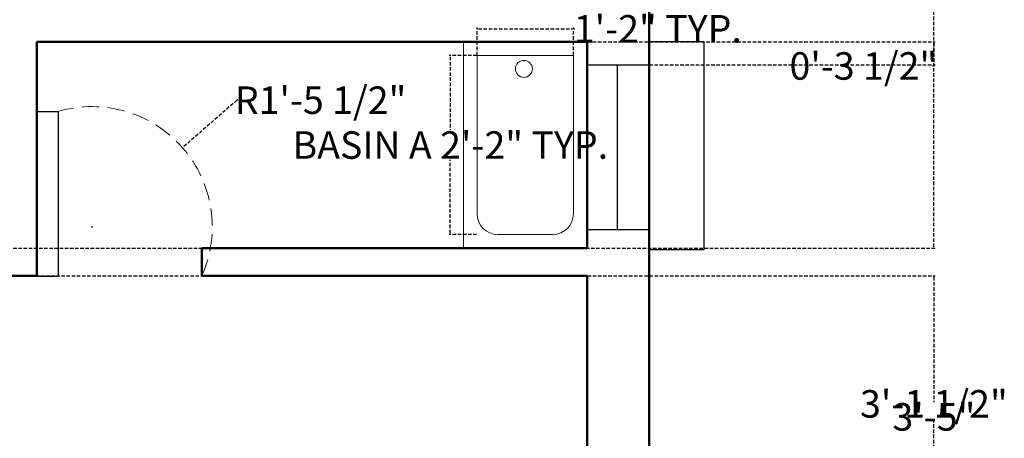
# Model space of a CAD drawing. Units: inches. Extents: x 513 to 1142, y 396 to 927.
# Tile 27 of 31: x 998 to 1142, y 614 to 674. Entities that reach past the tile are written whole.
import ezdxf

# ---------------------------------------------------------------- set-up
doc = ezdxf.new("R2010")
doc.units = ezdxf.units.IN
doc.header["$MEASUREMENT"] = 0
doc.linetypes.add('DASHED', pattern=[0.75, 0.5, -0.25])
for name, color, linetype, lineweight in [('A-ANNO-DIMS', 2, 'DASHED', 18), ('A-DOOR', 4, 'Continuous', 25), ('A-DOOR-SWNG', 4, 'DASHED', 13), ('A-FLOR-FIXT', 92, 'Continuous', 18), ('A-WALL', 7, 'Continuous', 50), ('windows', 172, 'Continuous', 25)]:
    doc.layers.add(name, color=color, linetype=linetype, lineweight=lineweight)
doc.styles.get("Standard").update_dxf_attribs({"font": 'arial.ttf'})
doc.dimstyles.get("Standard").update_dxf_attribs({"dimtxt": 4, "dimasz": 0.18, "dimexe": 0.18, "dimexo": 0.0625, "dimgap": 0.09, "dimtad": 0, "dimtih": 1, "dimtoh": 1, "dimdec": 0, "dimrnd": 6, "dimzin": 0, "dimdsep": 46, "dimlunit": 3, "dimtxsty": 'Standard', "dimcen": 0.09, "dimadec": 0, "dimazin": 0, "dimtfac": 1, "dimtdec": 0, "dimtofl": 0, "dimtmove": 0, "dimatfit": 3, "dimfxl": 1, "dimtolj": 1, "dimtzin": 0, "dimarcsym": 0})

# ---------------------------------------------------------------- blocks, each defined once
blk = doc.blocks.new('WIN-24IN')
blk.add_line((0, 4.39), (24, 4.39))
blk.add_lwpolyline([(24, 0), (0, 0), (0, 9), (24, 9)], close=True)
blk = doc.blocks.new('DOOR-LEAF-24IN')
blk.add_lwpolyline([(3, 24), (3, 0), (0, 0), (0, 24)], close=True)
blk = doc.blocks.new('BASIN-BOWL-14X26')
for p, q in [((0, 3), (0, 26)), ((0, 26), (14, 26)), ((14, 3), (14, 26)), ((3, 0), (11, 0))]:
    blk.add_line(p, q)
for centre, start, end in [((3, 3), 180, 270), ((11, 3), 270, 0)]:
    blk.add_arc(centre, 3, start, end)
blk = doc.blocks.new('*D131')
at = {"layer": 'A-ANNO-DIMS', "color": 0, "lineweight": -2, "transparency": 16777216}
for p, q in [((1064.93, 669.16), (1060.92, 669.16)), ((1061.1, 668.98), (1061.1, 658.32)), ((1061.1, 643.34), (1061.1, 654)), ((1064.93, 643.16), (1060.92, 643.16))]:
    blk.add_line(p, q, dxfattribs=at)
at = {"layer": 'A-ANNO-DIMS', "color": 0, "transparency": 16777216}
for points in [[(1061.07, 668.98), (1061.13, 668.98), (1061.1, 669.16)], [(1061.07, 643.34), (1061.13, 643.34), (1061.1, 643.16)]]:
    blk.add_solid(points, dxfattribs=at)
at = {"layer": 'Defpoints', "color": 0, "transparency": 16777216}
for p in [(1061.1, 669.16), (1065, 669.16), (1065, 643.16)]:
    blk.add_point(p, dxfattribs=at)
at = {"layer": 'A-ANNO-DIMS', "color": 0, "transparency": 16777216, "insert": (1061.1, 656.16), "char_height": 4, "attachment_point": 5}
blk.add_mtext('\\A1;BASIN A 2\'-2" TYP.', dxfattribs=at)
blk = doc.blocks.new('*D132')
at = {"layer": 'A-ANNO-DIMS', "color": 0, "lineweight": -2, "transparency": 16777216}
for p, q in [((1065, 669.22), (1065, 673.24)), ((1065.18, 673.06), (1078.82, 673.06)), ((1079, 669.22), (1079, 673.24)), ((1079, 673.06), (1079.18, 673.06))]:
    blk.add_line(p, q, dxfattribs=at)
at = {"layer": 'A-ANNO-DIMS', "color": 0, "transparency": 16777216}
for points in [[(1065.18, 673.09), (1065.18, 673.03), (1065, 673.06)], [(1078.82, 673.09), (1078.82, 673.03), (1079, 673.06)]]:
    blk.add_solid(points, dxfattribs=at)
at = {"layer": 'Defpoints', "color": 0, "transparency": 16777216}
for p in [(1079, 673.06), (1065, 669.16), (1079, 669.16)]:
    blk.add_point(p, dxfattribs=at)
at = {"layer": 'A-ANNO-DIMS', "color": 0, "transparency": 16777216, "insert": (1091.27, 673.06), "char_height": 4, "attachment_point": 5}
blk.add_mtext('\\A1;1\'-2" TYP.', dxfattribs=at)
blk = doc.blocks.new('*D149')
at = {"layer": 'A-ANNO-DIMS', "color": 0, "lineweight": -2, "transparency": 16777216}
for p, q in [((840.06, 770.16), (1131.58, 770.16)), ((1131.4, 769.98), (1131.4, 707.79)), ((1131.4, 641.34), (1131.4, 703.53)), ((840.06, 641.16), (1131.58, 641.16))]:
    blk.add_line(p, q, dxfattribs=at)
at = {"layer": 'A-ANNO-DIMS', "color": 0, "transparency": 16777216}
for points in [[(1131.37, 769.98), (1131.43, 769.98), (1131.4, 770.16)], [(1131.37, 641.34), (1131.43, 641.34), (1131.4, 641.16)]]:
    blk.add_solid(points, dxfattribs=at)
at = {"layer": 'Defpoints', "color": 0, "transparency": 16777216}
for p in [(840, 770.16), (1131.4, 770.16), (840, 641.16)]:
    blk.add_point(p, dxfattribs=at)
at = {"layer": 'A-ANNO-DIMS', "color": 0, "transparency": 16777216, "insert": (1131.4, 705.66), "char_height": 4, "attachment_point": 5}
blk.add_mtext('\\A1;10\'-9"', dxfattribs=at)
blk = doc.blocks.new('*D162')
at = {"layer": 'A-ANNO-DIMS', "color": 0, "lineweight": -2, "transparency": 16777216}
for p, q in [((1081.06, 637.16), (1131.58, 637.16)), ((1131.4, 636.98), (1131.4, 620.68)), ((1131.4, 600.06), (1131.4, 616.36)), ((1080.99, 599.88), (1131.58, 599.88))]:
    blk.add_line(p, q, dxfattribs=at)
at = {"layer": 'A-ANNO-DIMS', "color": 0, "transparency": 16777216}
for points in [[(1131.37, 636.98), (1131.43, 636.98), (1131.4, 637.16)], [(1131.37, 600.06), (1131.43, 600.06), (1131.4, 599.88)]]:
    blk.add_solid(points, dxfattribs=at)
at = {"layer": 'Defpoints', "color": 0, "transparency": 16777216}
for p in [(1081, 637.16), (1080.93, 599.88), (1131.4, 599.88)]:
    blk.add_point(p, dxfattribs=at)
at = {"layer": 'A-ANNO-DIMS', "color": 0, "transparency": 16777216, "insert": (1131.4, 618.52), "char_height": 4, "attachment_point": 5}
blk.add_mtext('\\A1;3\'-1 1/2"', dxfattribs=at)
blk = doc.blocks.new('*D166')
at = {"layer": 'A-ANNO-DIMS', "color": 0, "lineweight": -2, "transparency": 16777216}
for p, q in [((1081.06, 671.16), (1131.58, 671.16)), ((1131.4, 670.98), (1131.4, 668.02)), ((1081.03, 667.84), (1131.58, 667.84)), ((1131.4, 667.66), (1131.22, 667.66)), ((1131.4, 667.84), (1131.4, 667.66))]:
    blk.add_line(p, q, dxfattribs=at)
at = {"layer": 'A-ANNO-DIMS', "color": 0, "transparency": 16777216}
for points in [[(1131.37, 670.98), (1131.43, 670.98), (1131.4, 671.16)], [(1131.37, 668.02), (1131.43, 668.02), (1131.4, 667.84)]]:
    blk.add_solid(points, dxfattribs=at)
at = {"layer": 'Defpoints', "color": 0, "transparency": 16777216}
for p in [(1081, 671.16), (1080.97, 667.84), (1131.4, 667.84)]:
    blk.add_point(p, dxfattribs=at)
at = {"layer": 'A-ANNO-DIMS', "color": 0, "transparency": 16777216, "insert": (1121.15, 667.66), "char_height": 4, "attachment_point": 5}
blk.add_mtext('\\A1;0\'-3 1/2"', dxfattribs=at)
blk = doc.blocks.new('*D173')
at = {"layer": 'A-ANNO-DIMS', "color": 0, "lineweight": -2, "transparency": 16777216}
for p, q in [((904.06, 637.16), (1131.58, 637.16)), ((1131.4, 636.98), (1131.4, 618.76)), ((1131.4, 596.27), (1131.4, 614.49)), ((904.06, 596.09), (1131.58, 596.09))]:
    blk.add_line(p, q, dxfattribs=at)
at = {"layer": 'A-ANNO-DIMS', "color": 0, "transparency": 16777216}
for points in [[(1131.37, 636.98), (1131.43, 636.98), (1131.4, 637.16)], [(1131.37, 596.27), (1131.43, 596.27), (1131.4, 596.09)]]:
    blk.add_solid(points, dxfattribs=at)
at = {"layer": 'Defpoints', "color": 0, "transparency": 16777216}
for p in [(904, 637.16), (1131.4, 637.16), (904, 596.09)]:
    blk.add_point(p, dxfattribs=at)
at = {"layer": 'A-ANNO-DIMS', "color": 0, "transparency": 16777216, "insert": (1131.4, 616.63), "char_height": 4, "attachment_point": 5}
blk.add_mtext('\\A1;3\'-5"', dxfattribs=at)
blk = doc.blocks.new('*D189')
at = {"layer": 'A-ANNO-DIMS', "color": 0, "lineweight": -2, "transparency": 16777216}
for p, q in [((1030.08, 662.68), (1022.31, 655.89)), ((1030.26, 662.68), (1030.08, 662.68)), ((1008.92, 644.26), (1009.1, 644.26)), ((1009.01, 644.17), (1009.01, 644.35))]:
    blk.add_line(p, q, dxfattribs=at)
at = {"layer": 'A-ANNO-DIMS', "color": 0, "transparency": 16777216}
blk.add_solid([(1022.29, 655.91), (1022.33, 655.87), (1022.18, 655.77)], dxfattribs=at)
at = {"layer": 'Defpoints', "color": 0, "transparency": 16777216}
for p in [(1022.18, 655.77), (1009.01, 644.26)]:
    blk.add_point(p, dxfattribs=at)
at = {"layer": 'A-ANNO-DIMS', "color": 0, "transparency": 16777216, "insert": (1042.24, 662.68), "char_height": 4, "attachment_point": 5}
blk.add_mtext('\\A1;R1\'-5 1/2"', dxfattribs=at)

msp = doc.modelspace()

# ---------------------------------------------------------------- linework, layer by layer
at = {"layer": 'A-DOOR-SWNG', "ltscale": 5}
msp.add_arc((1009.01, 644.26), 17.49, 336.0483, 106.2786, dxfattribs=at)
at = {"layer": 'A-FLOR-FIXT'}
msp.add_line((1063, 641.16), (1063, 671.16), dxfattribs=at)
msp.add_circle((1071.8, 667.23), 1.23, dxfattribs=at)
at = {"layer": 'A-WALL'}
for p, q in [((1090, 431.16), (1090, 879.16)), ((1001, 637.16), (1001, 671.16)), ((1001, 671.16), (1081, 671.16)), ((1081, 641.16), (1081, 671.16)), ((1025, 637.16), (1025, 641.16)), ((1025, 641.16), (1081, 641.16)), ((949, 637.16), (1001, 637.16)), ((1025, 637.16), (1081, 637.16)), ((1081, 497.16), (1081, 637.16))]:
    msp.add_line(p, q, dxfattribs=at)
at = {"layer": 'windows'}
for p, q in [((1098, 671.16), (1090, 671.16)), ((1098, 640.92), (1098, 671.16)), ((1098, 640.92), (1090, 640.92))]:
    msp.add_line(p, q, dxfattribs=at)

# ---------------------------------------------------------------- block references
at = {"layer": 'A-DOOR'}
msp.add_blockref('DOOR-LEAF-24IN', (1001.11, 637.05), dxfattribs=at)
at = {"layer": 'A-FLOR-FIXT'}
msp.add_blockref('BASIN-BOWL-14X26', (1064.99, 643.16), dxfattribs=at)
at = {"layer": 'windows', "rotation": 270.0000000000006}
msp.add_blockref('WIN-24IN', (1080.97, 667.84), dxfattribs=at)

# ---------------------------------------------------------------- dimensions: what is measured, and where the dimension line sits
at = {"layer": 'A-ANNO-DIMS'}
for base, p1, p2, picture, middle in [((1131.4, 770.16), (840, 641.16), (840, 770.16), '*D149', (1131.4, 705.66)), ((1131.4, 667.84), (1081, 671.16), (1080.97, 667.84), '*D166', (1121.15, 667.66)), ((1131.4, 637.16), (904, 596.09), (904, 637.16), '*D173', (1131.4, 616.63)), ((1131.4, 599.88), (1081, 637.16), (1080.93, 599.88), '*D162', (1131.4, 618.52))]:
    dim = msp.add_linear_dim(base=base, p1=p1, p2=p2, angle=90, dimstyle='Standard', override={"dimdec": 1, "dimlfac": 1, "dimrnd": 0, "dimzin": 1, "dimdsep": 46, "dimlunit": 4, "dimfrac": 2}, dxfattribs=at)
    dim.commit()
    dim.dimension.update_dxf_attribs({"geometry": picture, "text_midpoint": middle})
dim = msp.add_linear_dim(base=(1079, 673.06), p1=(1065, 669.16), p2=(1079, 669.16), text='<> TYP.', dimstyle='Standard', override={"dimdec": 1, "dimlfac": 1, "dimrnd": 0, "dimzin": 1, "dimdsep": 46, "dimlunit": 4, "dimfrac": 2}, dxfattribs=at)
dim.commit()
dim.dimension.update_dxf_attribs({"geometry": '*D132', "text_midpoint": (1091.27, 673.06)})
dim = msp.add_radius_dim(center=(1009.01, 644.26), mpoint=(1022.18, 655.77), dimstyle='Standard', override={"dimdec": 1, "dimlfac": 1, "dimrnd": 0, "dimzin": 1, "dimdsep": 46, "dimlunit": 4, "dimfrac": 2}, dxfattribs=at)
dim.commit()
dim.dimension.update_dxf_attribs({"geometry": '*D189', "text_midpoint": (1042.24, 662.68), "dimtype": 164})
dim = msp.add_linear_dim(base=(1061.1, 669.16), p1=(1065, 643.16), p2=(1065, 669.16), angle=90, text='BASIN A <> TYP.', dimstyle='Standard', override={"dimdec": 1, "dimlfac": 1, "dimrnd": 0, "dimzin": 1, "dimdsep": 46, "dimlunit": 4, "dimfrac": 2}, dxfattribs=at)
dim.commit()
dim.dimension.update_dxf_attribs({"geometry": '*D131', "text_midpoint": (1061.1, 656.16)})

doc.saveas('drawing.dxf')
